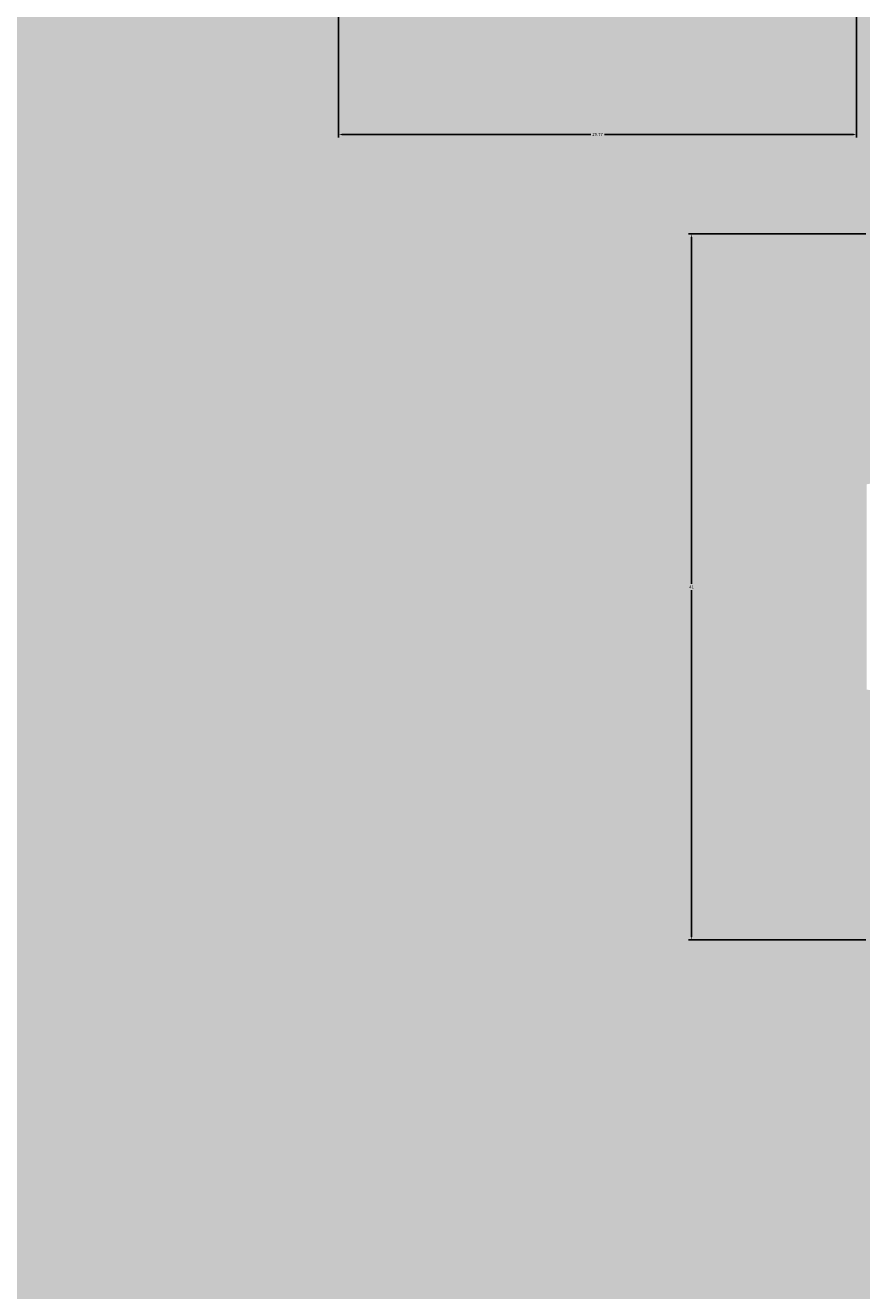
# Model space of a CAD drawing. Units: inches. Extents: x 3024 to 3952, y 1308 to 1863.
# Tile 6 of 29: x 3275 to 3323, y 1560 to 1633. Entities that reach past the tile are written whole.
import ezdxf

# ---------------------------------------------------------------- set-up
doc = ezdxf.new("R2010")
doc.units = ezdxf.units.IN
doc.layers.add('A-ANNO-DIMS', color=2, linetype='Continuous', lineweight=18)
doc.layers.add('A-FLOR-TILE-PATT', color=7, linetype='Continuous', lineweight=13)
doc.layers.add('A-FLOR-PATT', color=254, linetype='Continuous', lineweight=13, true_color=0xfeeab9)
doc.styles.get("Standard").update_dxf_attribs({"font": 'arial.ttf'})
doc.dimstyles.get("Standard").update_dxf_attribs({"dimtxt": 0.18, "dimasz": 0.18, "dimexe": 0.18, "dimexo": 0.0625, "dimgap": 0.09, "dimtad": 0, "dimtih": 1, "dimtoh": 1, "dimdec": 4, "dimzin": 0, "dimdsep": 46, "dimtxsty": 'Standard', "dimcen": 0.09, "dimadec": 0, "dimazin": 0, "dimtfac": 1, "dimtdec": 4, "dimtofl": 0, "dimtmove": 0, "dimatfit": 3, "dimfxl": 1, "dimtolj": 1, "dimtzin": 0, "dimarcsym": 0})

# ---------------------------------------------------------------- blocks, each defined once
blk = doc.blocks.new('*D21')
at = {"layer": 'A-ANNO-DIMS', "color": 0, "lineweight": -2, "transparency": 16777216}
for p, q in [((3323.055, 1621.114), (3312.873, 1621.114)), ((3313.053, 1620.934), (3313.053, 1601.018)), ((3313.053, 1580.742), (3313.053, 1600.657)), ((3323.055, 1580.562), (3312.873, 1580.562))]:
    blk.add_line(p, q, dxfattribs=at)
at = {"layer": 'A-ANNO-DIMS', "color": 0, "transparency": 16777216}
for points in [[(3313.023, 1620.934), (3313.083, 1620.934), (3313.053, 1621.114)], [(3313.023, 1580.742), (3313.083, 1580.742), (3313.053, 1580.562)]]:
    blk.add_solid(points, dxfattribs=at)
at = {"layer": 'Defpoints', "color": 0, "transparency": 16777216}
for p in [(3313.053, 1621.114), (3323.117, 1621.114), (3323.117, 1580.562)]:
    blk.add_point(p, dxfattribs=at)
at = {"layer": 'A-ANNO-DIMS', "color": 0, "transparency": 16777216, "insert": (3313.053, 1600.838), "char_height": 0.18, "attachment_point": 5}
blk.add_mtext('\\A1;41', dxfattribs=at)
blk = doc.blocks.new('*D63')
at = {"layer": 'A-ANNO-DIMS', "color": 0, "lineweight": -2, "transparency": 16777216}
for p, q in [((3292.764, 1652.544), (3292.764, 1626.651)), ((3322.536, 1652.544), (3322.536, 1626.651)), ((3292.944, 1626.831), (3307.255, 1626.831)), ((3322.356, 1626.831), (3308.045, 1626.831))]:
    blk.add_line(p, q, dxfattribs=at)
at = {"layer": 'A-ANNO-DIMS', "color": 0, "transparency": 16777216}
for points in [[(3292.944, 1626.861), (3292.944, 1626.801), (3292.764, 1626.831)], [(3322.356, 1626.861), (3322.356, 1626.801), (3322.536, 1626.831)]]:
    blk.add_solid(points, dxfattribs=at)
at = {"layer": 'Defpoints', "color": 0, "transparency": 16777216}
for p in [(3292.764, 1652.606), (3322.536, 1652.606), (3292.764, 1626.831)]:
    blk.add_point(p, dxfattribs=at)
at = {"layer": 'A-ANNO-DIMS', "color": 0, "transparency": 16777216, "insert": (3307.65, 1626.831), "char_height": 0.18, "attachment_point": 5}
blk.add_mtext('\\A1;29.77', dxfattribs=at)

msp = doc.modelspace()

# ---------------------------------------------------------------- hatches: boundary and pattern name
at = {"layer": 'A-FLOR-PATT', "transparency": 33554528}
h = msp.add_hatch(color=256, dxfattribs=at)
h.dxf.hatch_style = 1
h.paths.add_polyline_path([(3460.764, 1688.6064), (3412.764, 1688.6064), (3412.764, 1694.6064), (3460.764, 1694.6064), (3460.764, 1778.6064), (3406.764, 1778.6064), (3406.764, 1759.9514), (3318.2981, 1759.9514), (3318.2981, 1658.6064), (3322.5356, 1658.6064), (3322.5356, 1652.6064), (3292.764, 1652.6064), (3292.764, 1778.6064), (3106.764, 1778.6064), (3106.764, 1628.6064), (3172.764, 1628.6064), (3172.764, 1532.6064), (3166.764, 1532.6064), (3166.764, 1628.6064), (3106.764, 1628.6064), (3106.764, 1356.8452), (3202.812, 1356.8452), (3202.812, 1354.2534), (3202.812, 1353.8388), (3202.812, 1351.1212), (3202.812, 1347.8452), (3277.764, 1347.8452), (3277.764, 1353.8452), (3277.764, 1356.8452), (3277.764, 1442.6064), (3460.764, 1442.6064)])
h.paths.add_polyline_path([(3216.238, 1527.2064), (3216.238, 1491.2064), (3214.663, 1491.2064), (3214.663, 1491.2409, -0.3966224), (3180.243, 1526.6064), (3163.0285, 1526.6064), (3163.0285, 1531.1064), (3161.716, 1531.1064), (3161.716, 1561.1064), (3163.0285, 1561.1064), (3163.0285, 1531.1064), (3163.0285, 1526.6064), (3180.243, 1526.6064, 0.3966224), (3214.663, 1491.2409), (3214.663, 1527.2064)], flags=16)
h.paths.add_polyline_path([(3227.364, 1649.8972), (3191.364, 1649.8972), (3191.364, 1651.4722), (3227.364, 1651.4722)], flags=16)
h.paths.add_polyline_path([(3323.1172, 1606.7362), (3323.8545, 1606.8514), (3323.8545, 1594.8241), (3323.1172, 1594.9393)], flags=16)
h.paths.add_polyline_path([(3324.2232, 1606.909), (3330.1216, 1607.8307), (3330.1216, 1614.1093), (3339.3495, 1614.1093), (3340.2711, 1620.0078), (3352.4136, 1620.0078), (3353.3353, 1614.1093), (3359.9941, 1614.1093), (3360.9157, 1620.0078), (3373.0582, 1620.0078), (3373.9799, 1614.1093), (3383.2077, 1614.1093), (3383.2077, 1607.8307), (3389.1062, 1606.909), (3389.1062, 1594.7665), (3383.2077, 1593.8449), (3383.2077, 1587.5663), (3373.9799, 1587.5663), (3373.0583, 1581.6678), (3360.9157, 1581.6678), (3359.9941, 1587.5663), (3353.3353, 1587.5663), (3352.4136, 1581.6678), (3340.2711, 1581.6678), (3339.3495, 1587.5663), (3330.1216, 1587.5663), (3330.1216, 1593.8449), (3324.2232, 1594.7665)], flags=16)
h.paths.add_polyline_path([(3236.1584, 1693.1064), (3236.1584, 1723.1064), (3237.4709, 1723.1064), (3237.4709, 1693.1064)], flags=16)
h.paths.add_polyline_path([(3373.2158, 1600.6847), (3373.7965, 1600.7303), (3374.3268, 1600.7874), (3374.8132, 1600.8531), (3375.2621, 1600.9247), (3375.6801, 1600.9991), (3376.0736, 1601.0735), (3376.6855, 1601.19), (3377.366, 1601.3023), (3378.0667, 1601.3814), (3378.8026, 1601.4123), (3379.5865, 1601.3839), (3380.4537, 1601.2948), (3381.301, 1601.1717), (3382.0317, 1601.0433), (3382.4398, 1600.9607), (3382.6252, 1600.9201), (3382.919, 1600.8507), (3382.9044, 1600.8531), (3382.842, 1600.8678), (3382.7541, 1600.8896), (3382.6252, 1600.9201), (3382.4398, 1600.9607), (3382.1868, 1601.0119), (3381.8738, 1601.0711), (3381.5125, 1601.1346), (3381.1149, 1601.1988), (3380.6928, 1601.2601), (3380.2581, 1601.3149), (3379.8226, 1601.3597), (3379.3984, 1601.3908), (3378.9944, 1601.4054), (3378.6092, 1601.4042), (3378.2384, 1601.3886), (3377.8777, 1601.36), (3377.5227, 1601.32), (3377.1691, 1601.2698), (3376.8127, 1601.211), (3376.4491, 1601.145), (3376.0736, 1601.0735), (3375.4177, 1600.9494), (3374.5542, 1600.8119), (3373.5044, 1600.6988)], flags=0)
h.paths.add_polyline_path([(3380.0253, 1596.7351), (3380.499, 1596.6659), (3380.9706, 1596.6119), (3381.4375, 1596.5791), (3381.8971, 1596.5736), (3382.5886, 1596.6167), (3382.7848, 1596.6692), (3382.1465, 1596.5706), (3381.236, 1596.5815), (3380.3199, 1596.6865)], flags=0)
h.paths.add_polyline_path([(3369.6414, 1603.9617), (3370.1589, 1604.0021), (3370.6218, 1604.0539), (3371.0335, 1604.1173), (3371.3978, 1604.1921), (3371.7181, 1604.2785), (3371.9984, 1604.3761), (3372.2441, 1604.483), (3372.4611, 1604.5972), (3372.655, 1604.7163), (3372.8317, 1604.8384), (3372.9968, 1604.9611), (3373.3703, 1605.2455), (3373.8426, 1605.5328), (3374.4624, 1605.7539), (3375.1058, 1605.8302), (3375.7221, 1605.8261), (3376.4109, 1605.76), (3377.1534, 1605.6376), (3377.8945, 1605.473), (3378.1382, 1605.409), (3377.7394, 1605.5074), (3377.3509, 1605.5937), (3376.9704, 1605.6677), (3376.5999, 1605.7288), (3376.2417, 1605.7762), (3375.8979, 1605.8092), (3375.5707, 1605.8271), (3375.2621, 1605.8291), (3374.9745, 1605.8146), (3374.7092, 1605.7832), (3374.4647, 1605.7359), (3374.239, 1605.6742), (3374.0298, 1605.5996), (3373.835, 1605.5134), (3373.6525, 1605.4171), (3373.4801, 1605.3123), (3373.3156, 1605.2002), (3373.1562, 1605.0825), (3372.7603, 1604.781), (3372.236, 1604.4588), (3371.5738, 1604.2283), (3370.8493, 1604.0794), (3369.9262, 1603.976)], flags=0)
h.paths.add_polyline_path([(3366.7533, 1606.5832), (3367.1713, 1606.5519), (3367.5378, 1606.5374), (3367.8568, 1606.5394), (3368.1325, 1606.5573), (3368.3694, 1606.5903), (3368.5717, 1606.6377), (3368.7438, 1606.6988), (3368.89, 1606.7728), (3369.0146, 1606.8591), (3369.121, 1606.9568), (3369.2094, 1607.0646), (3369.2792, 1607.181), (3369.3295, 1607.3046), (3369.3596, 1607.4339), (3369.3688, 1607.5676), (3369.3565, 1607.7042), (3369.3218, 1607.8422), (3369.2649, 1607.9804), (3369.1893, 1608.1187), (3369.0993, 1608.2569), (3368.9992, 1608.3952), (3368.8934, 1608.5334), (3368.7861, 1608.6717), (3368.6817, 1608.8099), (3368.4212, 1609.1804), (3368.2685, 1609.7106), (3368.4883, 1610.1814), (3369.0537, 1610.4604), (3369.6717, 1610.5097), (3370.2812, 1610.3612), (3370.4805, 1610.2968), (3370.1882, 1610.3839), (3369.9284, 1610.4472), (3369.6905, 1610.4842), (3369.4662, 1610.4933), (3369.2555, 1610.4765), (3369.0608, 1610.4367), (3368.884, 1610.3767), (3368.7274, 1610.2994), (3368.5931, 1610.2077), (3368.4833, 1610.1045), (3368.4002, 1609.9927), (3368.3451, 1609.8747), (3368.3166, 1609.7517), (3368.3127, 1609.6244), (3368.331, 1609.4935), (3368.3696, 1609.3597), (3368.4261, 1609.2237), (3368.4985, 1609.0863), (3368.5845, 1608.9482), (3368.6817, 1608.8099), (3368.7861, 1608.6717), (3368.8934, 1608.5334), (3368.9992, 1608.3952), (3369.0993, 1608.2569), (3369.3398, 1607.8876), (3369.3941, 1607.2896), (3368.9774, 1606.7817), (3368.3928, 1606.5742), (3367.7162, 1606.5303), (3367.0044, 1606.5585)], flags=0)
h.paths.add_polyline_path([(3362.1859, 1610.2589), (3362.5478, 1610.2845), (3362.8348, 1610.3275), (3363.0585, 1610.3863), (3363.2303, 1610.4595), (3363.3619, 1610.5457), (3363.463, 1610.6432), (3363.5376, 1610.7502), (3363.5876, 1610.8643), (3363.6153, 1610.9834), (3363.6229, 1611.1055), (3363.6125, 1611.2283), (3363.5861, 1611.3496), (3363.5462, 1611.4673), (3363.4949, 1611.5797), (3363.4358, 1611.6871), (3363.3723, 1611.7902), (3363.3081, 1611.8897), (3363.2468, 1611.9863), (3363.192, 1612.0808), (3363.0258, 1612.4261), (3363.3371, 1612.8672), (3363.9008, 1612.9782), (3364.4822, 1612.9641), (3365.1098, 1612.9074), (3365.328, 1612.8805), (3364.9615, 1612.9208), (3364.6426, 1612.9496), (3364.3668, 1612.9669), (3364.1299, 1612.9726), (3363.9276, 1612.9669), (3363.7555, 1612.9496), (3363.6093, 1612.9208), (3363.4848, 1612.8805), (3363.3782, 1612.8289), (3363.2889, 1612.7672), (3363.2169, 1612.6969), (3363.1622, 1612.6193), (3363.1247, 1612.5361), (3363.1046, 1612.4484), (3363.1017, 1612.358), (3363.1161, 1612.266), (3363.1472, 1612.1738), (3363.192, 1612.0808), (3363.2468, 1611.9863), (3363.3081, 1611.8897), (3363.3723, 1611.7902), (3363.4358, 1611.6871), (3363.6363, 1611.323), (3363.5979, 1610.7003), (3363.0863, 1610.3651), (3362.3983, 1610.2622)], flags=0)
h.paths.add_polyline_path([(3352.356, 1581.2991), (3352.2408, 1580.5618), (3340.4439, 1580.5618), (3340.3287, 1581.2991)], flags=16)
h.paths.add_polyline_path([(3340.4439, 1621.1137), (3352.2408, 1621.1137), (3352.356, 1620.3764), (3340.3287, 1620.3764)], flags=16)
h.paths.add_polyline_path([(3278.4282, 1504.7424), (3290.3831, 1504.7424), (3290.3831, 1502.7499), (3291.0473, 1502.7499), (3291.0473, 1494.7799), (3290.3831, 1494.7799), (3290.3831, 1494.1158), (3291.0473, 1494.1158), (3291.0473, 1486.1458), (3290.3831, 1486.1458), (3290.3831, 1484.1533), (3291.0473, 1484.1533), (3291.0473, 1483.4892, -0.0909091), (3291.0473, 1468.8776), (3291.0473, 1468.2135), (3290.3831, 1468.2135), (3290.3831, 1464.8926), (3278.4282, 1464.8926), (3278.4282, 1472.8626), (3277.764, 1473.5268), (3277.764, 1478.84), (3278.4282, 1479.5042)], flags=16)
h.paths.add_polyline_path([(3278.7603, 1504.4103), (3290.051, 1504.4103), (3290.051, 1465.2247), (3278.7603, 1465.2247)], flags=0)
h.paths.add_polyline_path([(3123.904, 1600.7821), (3117.9039, 1602.7821), (3117.9039, 1599.7821), (3119.4039, 1599.7821), (3119.4039, 1596.7821), (3118.4039, 1596.7821), (3118.4039, 1598.7821), (3117.9039, 1598.7821), (3117.9039, 1596.2821), (3109.9039, 1596.2821), (3109.9039, 1617.2821), (3117.9039, 1617.2821), (3117.9039, 1610.7821), (3123.9038, 1612.7821, -0.7025712), (3137.9039, 1606.7822, -0.7025621)], flags=16)
h.paths.add_polyline_path([(3123.9039, 1602.7822), (3123.9039, 1610.7822, -0.7345333), (3136.9039, 1606.7822, -0.7345297)], flags=0)
h.paths.add_polyline_path([(3177.972, 1689.6473), (3109.2405, 1689.6473), (3109.2405, 1741.1959), (3177.972, 1741.1959)], flags=16)
h.paths.add_polyline_path([(3373.0006, 1581.2991), (3372.8854, 1580.5618), (3361.0885, 1580.5618), (3360.9733, 1581.2991)], flags=16)
h.paths.add_polyline_path([(3361.0885, 1621.1137), (3372.8854, 1621.1137), (3373.0006, 1620.3764), (3360.9733, 1620.3764)], flags=16)
h.paths.add_polyline_path([(3116.9039, 1598.2821, -0.4142136), (3116.1539, 1597.2821), (3111.9039, 1597.2821, -0.4142136), (3110.9039, 1598.0321), (3110.9039, 1615.2821, -0.4142136), (3111.6539, 1616.2821), (3115.9039, 1616.2821, -0.4142136), (3116.9039, 1615.5321)], flags=0)
h.paths.add_polyline_path([(3121.6122, 1728.1369), (3121.6122, 1696.5205), (3110.2715, 1696.5205), (3110.2715, 1714.3906), (3121.6122, 1714.3906), (3121.6122, 1716.4526), (3110.2715, 1716.4526), (3110.2715, 1734.3228), (3123.3304, 1734.3228), (3123.3304, 1729.8552), (3134.6711, 1741.1959), (3134.6711, 1728.1369)], flags=0)
h.paths.add_polyline_path([(3389.4748, 1606.8514), (3390.2122, 1606.7362), (3390.2122, 1594.9393), (3389.4748, 1594.8241)], flags=16)
h.paths.add_polyline_path([(3257.6842, 1762.8281), (3259.6842, 1768.8281), (3256.6842, 1768.8281), (3256.6842, 1767.3281), (3253.6842, 1767.3281), (3253.6842, 1768.3281), (3255.6842, 1768.3281), (3255.6842, 1768.8281), (3253.1842, 1768.8281), (3253.1842, 1776.8281), (3274.1842, 1776.8281), (3274.1842, 1768.8281), (3267.6842, 1768.8281), (3269.6842, 1762.8282, -0.7025712), (3263.6843, 1748.8282, -0.7025621)], flags=16)
h.paths.add_polyline_path([(3259.6842, 1762.8281), (3267.6843, 1762.8281, -0.7345333), (3263.6842, 1749.8282, -0.7345297)], flags=0)
h.paths.add_polyline_path([(3411.264, 1715.6064), (3411.264, 1716.9189), (3441.264, 1716.9189), (3441.264, 1715.6064)], flags=16)
h.paths.add_polyline_path([(3178.3806, 1449.1876), (3178.3806, 1397.639), (3109.6491, 1397.639), (3109.6491, 1449.1876)], flags=16)
h.paths.add_polyline_path([(3397.1501, 1541.7146), (3419.6183, 1541.7146), (3419.6183, 1496.7783), (3397.1501, 1496.7783)], flags=16)
h.paths.add_polyline_path([(3254.1842, 1770.5781), (3254.1842, 1774.8281, -0.4142136), (3254.9342, 1775.8281), (3272.1842, 1775.8281, -0.4142136), (3273.1842, 1775.0781), (3273.1842, 1770.8281, -0.4142136), (3272.4342, 1769.8281), (3255.1842, 1769.8281, -0.4142136)], flags=0)
h.paths.add_polyline_path([(3403.672, 1500.7601), (3403.6016, 1500.3997), (3403.5328, 1500.0441), (3403.4662, 1499.6867), (3403.4027, 1499.3226), (3403.3464, 1498.9532), (3403.3025, 1498.5811), (3403.2759, 1498.2091), (3403.2714, 1497.8401), (3403.3064, 1497.2813), (3403.3491, 1497.1219), (3403.2689, 1497.6395), (3403.2778, 1498.3719), (3403.3635, 1499.0984), (3403.4889, 1499.8168), (3403.6016, 1500.3997), (3403.672, 1500.7601), (3403.744, 1501.1315), (3403.817, 1501.5205), (3403.891, 1501.9336), (3403.9656, 1502.3769), (3404.0404, 1502.8572), (3404.115, 1503.3786), (3404.2264, 1504.2311), (3404.2571, 1504.5223), (3404.1552, 1503.6598), (3404.0063, 1502.6193), (3403.8604, 1501.7518), (3403.744, 1501.1315)], flags=0)
h.paths.add_polyline_path([(3406.5868, 1505.0416), (3406.6121, 1504.5236), (3406.6492, 1504.0526), (3406.6956, 1503.624), (3406.7491, 1503.2333), (3406.8072, 1502.8759), (3406.8676, 1502.5473), (3406.9281, 1502.243), (3407.0268, 1501.7597), (3407.1416, 1501.1368), (3407.2087, 1500.3904), (3407.1804, 1499.6703), (3407.1078, 1498.9956), (3407.0074, 1498.3199), (3406.8809, 1497.6059), (3406.7403, 1496.9627), (3406.7418, 1496.9824), (3406.7491, 1497.0249), (3406.8229, 1497.3409), (3406.8364, 1497.4025), (3406.878, 1497.6078), (3406.9261, 1497.8614), (3406.9777, 1498.1526), (3407.0298, 1498.4712), (3407.0797, 1498.8068), (3407.1243, 1499.149), (3407.1607, 1499.4874), (3407.1859, 1499.8115), (3407.1978, 1500.1137), (3407.1969, 1500.3962), (3407.1841, 1500.6642), (3407.1609, 1500.9225), (3407.1284, 1501.1761), (3407.0876, 1501.43), (3407.0398, 1501.6891), (3406.9862, 1501.9585), (3406.8832, 1502.4628), (3406.7712, 1503.0713), (3406.6657, 1503.8424), (3406.5924, 1504.7735)], flags=0)
h.paths.add_polyline_path([(3409.2517, 1507.8962), (3409.2752, 1507.4282), (3409.3079, 1507.0076), (3409.3501, 1506.6314), (3409.4015, 1506.2969), (3409.4624, 1506.0009), (3409.5326, 1505.7406), (3409.6119, 1505.5128), (3409.6988, 1505.3131), (3409.7915, 1505.1368), (3409.8883, 1504.9792), (3409.9875, 1504.8356), (3410.0872, 1504.7015), (3410.1859, 1504.572), (3410.4508, 1504.2132), (3410.7205, 1503.6035), (3410.8059, 1502.8824), (3410.7619, 1502.0875), (3410.6122, 1501.2299), (3410.4402, 1500.6169), (3410.2538, 1500.0031), (3410.0536, 1499.3219), (3409.9909, 1499.0812), (3410.1761, 1499.7472), (3410.3596, 1500.3513), (3410.4512, 1500.6561), (3410.5312, 1500.9412), (3410.6013, 1501.226), (3410.6614, 1501.512), (3410.7111, 1501.7964), (3410.7496, 1502.0763), (3410.7764, 1502.3489), (3410.7909, 1502.6114), (3410.7926, 1502.8608), (3410.7808, 1503.0944), (3410.7553, 1503.31), (3410.7169, 1503.5087), (3410.6667, 1503.6921), (3410.6061, 1503.8621), (3410.5361, 1504.0203), (3410.4578, 1504.1686), (3410.3726, 1504.3088), (3410.2815, 1504.4424), (3410.1859, 1504.572), (3410.0872, 1504.7015), (3409.859, 1505.0083), (3409.5943, 1505.5117), (3409.4266, 1506.1336), (3409.324, 1506.8011), (3409.2586, 1507.6407)], flags=0)
h.paths.add_polyline_path([(3411.4914, 1510.5878), (3411.4432, 1510.1586), (3411.4054, 1509.775), (3411.38, 1509.4354), (3411.3681, 1509.1376), (3411.3698, 1508.8784), (3411.3843, 1508.6542), (3411.4112, 1508.4618), (3411.4497, 1508.2974), (3411.4994, 1508.1575), (3411.5595, 1508.0388), (3411.6296, 1507.9375), (3411.7097, 1507.851), (3411.802, 1507.7792), (3411.9096, 1507.7225), (3412.0353, 1507.6817), (3412.1821, 1507.6572), (3412.3528, 1507.6496), (3412.5505, 1507.6597), (3412.778, 1507.6879), (3413.0364, 1507.7341), (3413.3194, 1507.7955), (3413.6188, 1507.8687), (3413.9264, 1507.95), (3414.234, 1508.036), (3414.5333, 1508.1232), (3414.8163, 1508.208), (3415.0747, 1508.287), (3415.3023, 1508.3569), (3415.5007, 1508.4158), (3415.6733, 1508.4617), (3416.1158, 1508.5538), (3416.512, 1508.2591), (3416.716, 1507.6581), (3416.61, 1507.0003), (3416.3052, 1506.3411), (3415.8928, 1505.618), (3415.7339, 1505.3633), (3415.9914, 1505.791), (3416.201, 1506.1583), (3416.3666, 1506.4739), (3416.4925, 1506.7462), (3416.5828, 1506.9838), (3416.6413, 1507.1949), (3416.6725, 1507.3883), (3416.6799, 1507.5705), (3416.6662, 1507.7417), (3416.6339, 1507.9), (3416.5851, 1508.0436), (3416.5223, 1508.1709), (3416.4478, 1508.28), (3416.3639, 1508.3692), (3416.273, 1508.4368), (3416.1765, 1508.4815), (3416.0718, 1508.5047), (3415.9553, 1508.5079), (3415.8237, 1508.493), (3415.6733, 1508.4617), (3415.5007, 1508.4158), (3415.3327, 1508.3659), (3414.6495, 1508.157), (3414.0606, 1507.9855), (3413.4456, 1507.8229), (3412.8838, 1507.701), (3412.5505, 1507.6597), (3412.0748, 1507.6354), (3411.595, 1507.8883), (3411.398, 1508.4429), (3411.3624, 1508.9927), (3411.3854, 1509.5711), (3411.4578, 1510.3071)], flags=0)
h.paths.add_polyline_path([(3135.0797, 1449.1876), (3135.0797, 1436.1286), (3122.0208, 1436.1286), (3122.0208, 1404.5122), (3110.6801, 1404.5122), (3110.6801, 1422.3823), (3122.0208, 1422.3823), (3122.0208, 1424.4443), (3110.6801, 1424.4443), (3110.6801, 1442.3145), (3123.739, 1442.3145), (3123.739, 1437.8469)], flags=0)
h.paths.add_polyline_path([(3416.4944, 1514.2949), (3416.4837, 1513.8511), (3416.4893, 1513.4867), (3416.5102, 1513.1926), (3416.5451, 1512.9593), (3416.5929, 1512.7775), (3416.6524, 1512.6379), (3416.7224, 1512.531), (3416.8017, 1512.4488), (3416.8886, 1512.3882), (3416.9813, 1512.3476), (3417.0781, 1512.3251), (3417.1773, 1512.3189), (3417.277, 1512.3274), (3417.3757, 1512.3488), (3417.4713, 1512.3813), (3417.5627, 1512.4229), (3417.65, 1512.471), (3417.7338, 1512.5225), (3417.8146, 1512.5747), (3417.8931, 1512.6245), (3417.9699, 1512.6691), (3418.2968, 1512.8265), (3418.6505, 1512.4645), (3418.7037, 1511.9342), (3418.6693, 1511.3839), (3418.6076, 1510.8228), (3418.5777, 1510.5927), (3418.6197, 1510.9333), (3418.6525, 1511.2311), (3418.6759, 1511.4903), (3418.6899, 1511.7144), (3418.6946, 1511.9069), (3418.6899, 1512.0713), (3418.6759, 1512.2112), (3418.6525, 1512.33), (3418.6197, 1512.4311), (3418.5778, 1512.5177), (3418.5276, 1512.5903), (3418.4705, 1512.6488), (3418.4075, 1512.6933), (3418.3399, 1512.7237), (3418.2686, 1512.7401), (3418.1951, 1512.7424), (3418.1204, 1512.7307), (3418.0455, 1512.7055), (3417.9792, 1512.6736), (3417.65, 1512.471), (3417.5627, 1512.4229), (3417.4713, 1512.3813), (3417.3757, 1512.3488), (3417.277, 1512.3274), (3416.878, 1512.2936), (3416.5757, 1512.7549), (3416.492, 1513.3145), (3416.4808, 1514.0384)], flags=0)
h.paths.add_polyline_path([(3392.8223, 1481.9454), (3396.7707, 1481.9454), (3396.7707, 1480.9201), (3428.3585, 1480.9201), (3428.3585, 1481.9454), (3432.3069, 1481.9454), (3432.3069, 1464.8354, -0.266667), (3392.8223, 1464.8354)], flags=16)
h.paths.add_polyline_path([(3431.203, 1547.5428), (3450.8613, 1547.5428, -0.1904762), (3450.8614, 1484.031), (3431.203, 1484.031), (3431.203, 1488.5675), (3432.3809, 1488.5675), (3432.3809, 1543.0062), (3431.203, 1543.0062)], flags=16)
h.paths.add_polyline_path([(3451.9233, 1524.86, -0.0496282), (3451.9233, 1506.7138), (3446.7921, 1506.7138), (3446.7921, 1524.86)], flags=0)
h.paths.add_polyline_path([(3460.764, 1436.6064), (3277.764, 1436.6064), (3277.764, 1356.8452), (3277.764, 1353.8452), (3460.764, 1353.8452)], flags=17)
h.paths.add_polyline_path([(3121.3033, 1577.378), (3153.693, 1577.378), (3153.693, 1586.6752), (3121.3033, 1586.6752)], flags=24)
h.paths.add_polyline_path([(3164.1457, 1464.1276), (3210.4801, 1464.1276), (3210.4801, 1473.4247), (3164.1457, 1473.4247)], flags=24)
h.paths.add_polyline_path([(3343.1909, 1505.8863), (3373.7236, 1505.8863), (3373.7236, 1515.1773), (3343.1909, 1515.1773)], flags=24)
h.paths.add_polyline_path([(3337.6353, 1564.2926), (3370.0189, 1564.2926), (3370.0189, 1573.5836), (3337.6353, 1573.5836)], flags=24)
h.paths.add_polyline_path([(3419.204, 1753.8578), (3453.3997, 1753.8578), (3453.3997, 1762.9956), (3419.204, 1762.9956)], flags=24)
h.paths.add_polyline_path([(3341.2523, 1701.0246), (3381.0761, 1701.0246), (3381.0761, 1710.3156), (3341.2523, 1710.3156)], flags=24)
h.paths.add_polyline_path([(3245.8895, 1726.2997), (3278.2793, 1726.2997), (3278.2793, 1735.5968), (3245.8895, 1735.5968)], flags=24)
h.paths.add_polyline_path([(3128.8045, 1668.6736), (3175.1389, 1668.6736), (3175.1389, 1677.9707), (3128.8045, 1677.9707)], flags=24)
h.paths.add_polyline_path([(3345.9997, 1396.0062), (3389.09, 1396.0062), (3389.09, 1405.3033), (3345.9997, 1405.3033)], flags=24)
at = {"layer": 'A-FLOR-TILE-PATT', "transparency": 33554569}
h = msp.add_hatch(dxfattribs=at)
h.set_pattern_fill('ANGLE', color=256, scale=2)
h.set_pattern_definition([(0, (0, 0), (0, 13.97), [10.16, -3.81]), (90, (0, 0), (-13.97, 9e-16), [10.16, -3.81])])
h.paths.add_polyline_path([(3292.764, 1778.6064), (3232.764, 1778.6064), (3232.764, 1694.6064), (3236.1584, 1694.6064), (3236.1584, 1723.1064), (3237.4709, 1723.1064), (3237.4709, 1723.0777, -0.3870039), (3266.1209, 1694.6064), (3292.764, 1694.6064)])
h.paths.add_polyline_path([(3263.6843, 1748.8282, -0.7025621), (3257.6842, 1762.8281), (3259.6842, 1768.8281), (3256.6842, 1768.8281), (3256.6842, 1767.3281), (3253.6842, 1767.3281), (3253.6842, 1768.3281), (3255.6842, 1768.3281), (3255.6842, 1768.8281), (3253.1842, 1768.8281), (3253.1842, 1776.8281), (3274.1842, 1776.8281), (3274.1842, 1768.8281), (3267.6842, 1768.8281), (3269.6842, 1762.8282, -0.7025712)], flags=16)
h.paths.add_polyline_path([(3263.6842, 1749.8282, -0.7345297), (3259.6842, 1762.8281), (3267.6843, 1762.8281, -0.7345333)], flags=0)
h.paths.add_polyline_path([(3255.1842, 1769.8281, -0.4142136), (3254.1842, 1770.5781), (3254.1842, 1774.8281, -0.4142136), (3254.9342, 1775.8281), (3272.1842, 1775.8281, -0.4142136), (3273.1842, 1775.0781), (3273.1842, 1770.8281, -0.4142136), (3272.4342, 1769.8281)], flags=0)
h.paths.add_polyline_path([(3460.764, 1436.6064), (3277.764, 1436.6064), (3277.764, 1356.8452), (3277.764, 1353.8452), (3460.764, 1353.8452)])
h.paths.add_polyline_path([(3166.764, 1628.6064), (3106.764, 1628.6064), (3106.764, 1532.6064), (3133.066, 1532.6064, -0.3870039), (3161.716, 1561.0777), (3161.716, 1561.1064), (3163.0285, 1561.1064), (3163.0285, 1532.6064), (3166.764, 1532.6064)])
h.paths.add_polyline_path([(3123.904, 1600.7821), (3117.9039, 1602.7821), (3117.9039, 1599.7821), (3119.4039, 1599.7821), (3119.4039, 1596.7821), (3118.4039, 1596.7821), (3118.4039, 1598.7821), (3117.9039, 1598.7821), (3117.9039, 1596.2821), (3109.9039, 1596.2821), (3109.9039, 1617.2821), (3117.9039, 1617.2821), (3117.9039, 1610.7821), (3123.9038, 1612.7821, -0.7025712), (3137.9039, 1606.7822, -0.7025621)], flags=16)
h.paths.add_polyline_path([(3123.9039, 1602.7822), (3123.9039, 1610.7822, -0.7345333), (3136.9039, 1606.7822, -0.7345297)], flags=0)
h.paths.add_polyline_path([(3116.1539, 1597.2821), (3111.9039, 1597.2821, -0.4142136), (3110.9039, 1598.0321), (3110.9039, 1615.2821, -0.4142136), (3111.6539, 1616.2821), (3115.9039, 1616.2821, -0.4142136), (3116.9039, 1615.5321), (3116.9039, 1598.2821, -0.4142136)], flags=0)
h.paths.add_polyline_path([(3245.8895, 1726.2997), (3278.2793, 1726.2997), (3278.2793, 1735.5968), (3245.8895, 1735.5968)], flags=24)
h.paths.add_polyline_path([(3345.9997, 1396.0062), (3389.09, 1396.0062), (3389.09, 1405.3033), (3345.9997, 1405.3033)], flags=24)
h.paths.add_polyline_path([(3121.3033, 1577.378), (3153.693, 1577.378), (3153.693, 1586.6752), (3121.3033, 1586.6752)], flags=24)

# ---------------------------------------------------------------- dimensions: what is measured, and where the dimension line sits
at = {"layer": 'A-ANNO-DIMS'}
for base, p1, p2, angle, override, picture, middle in [((3292.764, 1626.8314), (3322.5356, 1652.6064), (3292.764, 1652.6064), 180, {"dimdec": 2, "dimlfac": 1, "dimrnd": 0, "dimzin": 0, "dimdsep": 46, "dimlunit": 2}, '*D63', (3307.6498, 1626.8314)), ((3313.053, 1621.1137), (3323.1172, 1580.5618), (3323.1172, 1621.1137), 90, {"dimdec": 0, "dimlfac": 1, "dimrnd": 0, "dimzin": 0, "dimdsep": 46, "dimlunit": 2}, '*D21', (3313.053, 1600.8378))]:
    dim = msp.add_linear_dim(base=base, p1=p1, p2=p2, angle=angle, dimstyle='Standard', override=override, dxfattribs=at)
    dim.commit()
    dim.dimension.update_dxf_attribs({"geometry": picture, "text_midpoint": middle})

doc.saveas('drawing.dxf')
